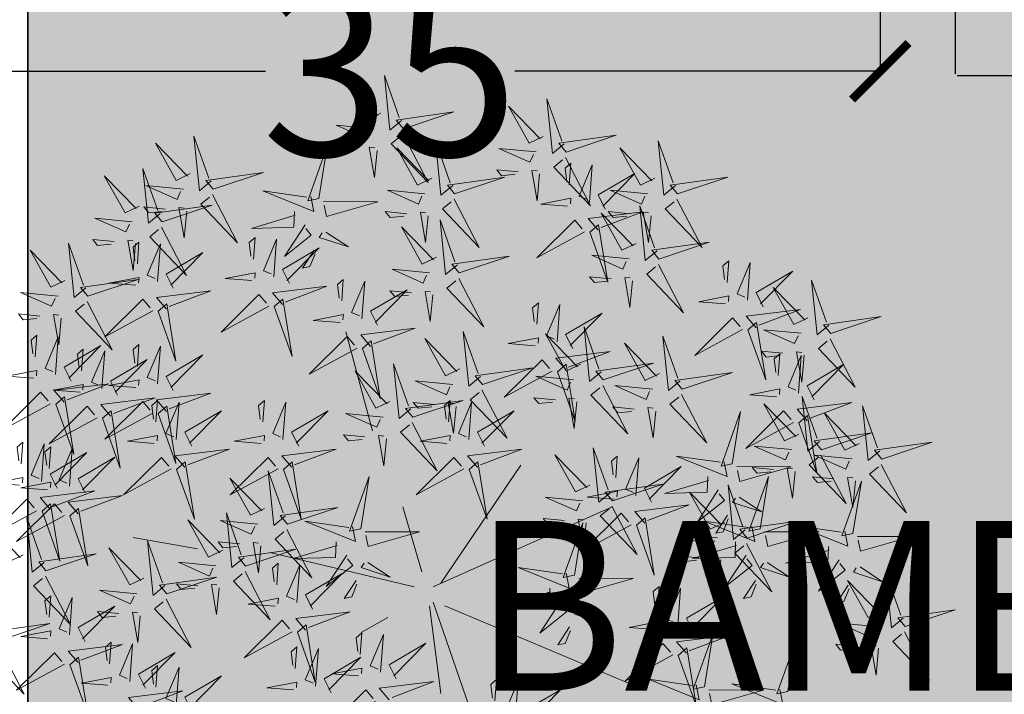
# Model space of a CAD drawing. Units: inches. Extents: x 1704 to 6393, y -157 to 1172.
# Tile 4 of 122: x 1898 to 1933, y 17 to 41. Entities that reach past the tile are written whole.
import ezdxf

# ---------------------------------------------------------------- set-up
doc = ezdxf.new("R2010")
doc.units = ezdxf.units.IN
doc.header["$MEASUREMENT"] = 0
for name, color, linetype, lineweight in [('A-ANNO-DIMS', 7, 'Continuous', 13), ('C-PROP', 7, 'Continuous', 35), ('L-shrub', 74, 'Continuous', 18), ('L-tree', 102, 'Continuous', 18)]:
    doc.layers.add(name, color=color, linetype=linetype, lineweight=lineweight)
doc.layers.add('L-PLNT-PATT', color=253, linetype='Continuous', lineweight=13, true_color=0x9abc8f)
doc.styles.get("Standard").update_dxf_attribs({"font": 'arial.ttf'})
doc.dimstyles.get("Standard").update_dxf_attribs({"dimtxt": 6, "dimasz": 2, "dimexe": 0.18, "dimexo": 0.0625, "dimgap": 0.09, "dimtad": 0, "dimtih": 1, "dimtoh": 1, "dimdec": 1, "dimzin": 0, "dimdsep": 46, "dimlunit": 3, "dimtxsty": 'Standard', "dimblk": 'ARCHTICK', "dimcen": 0.09, "dimadec": 0, "dimazin": 0, "dimtfac": 1, "dimtdec": 1, "dimtofl": 0, "dimtmove": 0, "dimatfit": 3, "dimfxl": 1, "dimtolj": 1, "dimtzin": 0, "dimarcsym": 0})

# ---------------------------------------------------------------- blocks, each defined once
blk = doc.blocks.new('bamboo')
at = {"layer": 'L-shrub'}
for p, q in [((43.5, 73), (278.2, 631.2)), ((-12.4, 39.5), (-247.1, 564.2)), ((-23.6, 61.9), (-370, 296.3)), ((32.3, 39.5), (390, 162.3)), ((43.5, 28.4), (300.5, 61.9)), ((-57.1, 6), (-247.1, -49.8)), ((-12.4, -16.3), (-113, -440.5)), ((77, -94.4), (121.7, -172.6)), ((-470.6, -139.1), (-761.2, -217.2)), ((-124.2, -652.6), (-157.7, -842.3))]:
    blk.add_line(p, q, dxfattribs=at)
for points in [[(103.7, 1424.7), (54.4, 1572.3), (77.9, 1403.4), (103.7, 1424.7)], [(-387.8, 1356.5), (-437.1, 1504.1), (-413.6, 1335.2), (-387.8, 1356.5)], [(119.4, 1423.2), (261.4, 1496.7), (147.9, 1388.7), (126.6, 1414.5)], [(-372, 1355), (-230.1, 1428.5), (-343.6, 1320.5), (-364.9, 1346.4)], [(-160.7, 1284.9), (-160, 1444.8), (-116.9, 1294.1), (-149.7, 1287.2)], [(79.4, 1419.1), (107.8, 1384.6), (-52.4, 1368.4), (70.8, 1412)], [(-756.4, 1206.5), (-805.8, 1354.1), (-782.2, 1185.2), (-756.4, 1206.5)], [(-412.1, 1350.9), (-383.7, 1316.4), (-543.9, 1300.2), (-420.7, 1343.8)], [(-70.9, 1292.4), (-27.7, 1358.5), (-55.4, 1272.9), (-68.6, 1281.5)], [(57.7, 1357.7), (77.5, 1316.1), (-31.5, 1255.3), (64.8, 1349.1)], [(103.3, 1337.4), (92.8, 1227.4), (133.3, 1318.7), (110.4, 1328.8)], [(167.7, 1347.1), (246.3, 1339.5), (157.6, 1324.2), (159.1, 1340)], [(-415.1, 1179.2), (-464.4, 1326.8), (-440.9, 1157.9), (-415.1, 1179.2)], [(-740.7, 1205), (-598.8, 1278.5), (-712.2, 1170.5), (-733.6, 1196.4)], [(-433.8, 1289.5), (-414, 1248), (-523, 1187.1), (-426.7, 1280.9)], [(-323.8, 1278.9), (-245.2, 1271.3), (-333.9, 1256.1), (-332.4, 1271.8)], [(-169.3, 1271.7), (-323, 1296.4), (-162.4, 1238.9), (-169.3, 1271.7)], [(161.7, 1284.2), (155.7, 1221.3), (172.9, 1235.5), (168.8, 1275.6)], [(-561.9, 1157.8), (-603.1, 1137.1), (-666.2, 1244.8), (-570.4, 1150.5)], [(-500.1, 1137.3), (-534, 1108.2), (-553.5, 1268), (-507.4, 1145.8)], [(-399.4, 1177.7), (-257.4, 1251.3), (-370.9, 1143.2), (-392.2, 1169.1)], [(-388.2, 1269.3), (-398.7, 1159.2), (-358.2, 1250.5), (-381.1, 1260.6)], [(-175.7, 1247.6), (-131.9, 1256.8), (-191.9, 1107.3), (-173.4, 1236.6)], [(-92.2, 1230.9), (0.4, 1170.5), (-61.7, 1248.7), (-81.3, 1233.2)], [(-18, 1257.9), (35, 1223.4), (30.4, 1245.3), (-7, 1260.2)], [(-329.8, 1216), (-335.8, 1153.1), (-318.6, 1167.3), (-322.7, 1207.4)], [(-780.7, 1200.9), (-752.3, 1166.4), (-912.5, 1150.2), (-789.3, 1193.8)], [(-131.4, 1199.8), (-85.3, 1198.1), (-81.9, 1073.4), (-120.4, 1202.1)], [(-439.4, 1173.7), (-411, 1139.2), (-571.2, 1122.9), (-448, 1166.6)], [(-494, 1113.1), (-347.5, 1165.5), (-515.9, 1138.5), (-494, 1113.1)], [(-174.3, 1012.2), (-173.7, 1172.1), (-130.6, 1021.4), (-163.4, 1014.5)], [(-802.5, 1139.6), (-782.6, 1098), (-891.6, 1037.1), (-795.3, 1130.9)], [(-692.4, 1128.9), (-613.8, 1121.3), (-702.5, 1106.1), (-701, 1121.8)], [(-773.2, 987.3), (-807.1, 958.2), (-826.6, 1118), (-780.4, 995.8)], [(-756.8, 1119.3), (-767.3, 1009.2), (-726.8, 1100.5), (-749.7, 1110.6)], [(-581.3, 1111.7), (-691.5, 1120), (-599.4, 1081.4), (-589.8, 1104.4)], [(-461.1, 1112.3), (-441.3, 1070.7), (-550.3, 1009.8), (-454, 1103.7)], [(-351.1, 1101.6), (-272.5, 1094), (-361.2, 1078.8), (-359.7, 1094.5)], [(-155.7, 961.1), (-205, 1108.7), (-181.5, 939.8), (-155.7, 961.1)], [(294.9, 1080.8), (141.2, 1105.5), (301.8, 1048), (294.9, 1080.8)], [(-835, 1007.8), (-876.2, 987.1), (-939.2, 1094.8), (-843.4, 1000.5)], [(-495.2, 1097.3), (-418.8, 957), (-529.1, 1068.2), (-503.7, 1090.1)], [(-415.5, 1092), (-426, 981.9), (-385.5, 1073.2), (-408.4, 1083.4)], [(-365.5, 930.4), (-364.8, 1090.2), (-321.7, 939.6), (-354.5, 932.7)], [(-84.5, 1019.7), (-41.3, 1085.8), (-69, 1000.1), (-82.2, 1008.8)], [(-698.4, 1066), (-704.4, 1003.1), (-687.2, 1017.3), (-691.3, 1057.4)], [(-633.3, 1052.3), (-696.3, 1057), (-681.8, 1040.1), (-641.8, 1045)], [(-570.3, 1047.5), (-576.3, 968.8), (-593.4, 1057.2), (-577.6, 1056)], [(288.5, 1056.7), (332.3, 1065.9), (272.3, 916.4), (290.8, 1045.7)], [(-767.1, 963.1), (-620.5, 1015.5), (-788.9, 988.5), (-767.1, 963.1)], [(-357.1, 1038.7), (-363.1, 975.8), (-345.9, 990), (-350, 1030.1)], [(-183, 999), (-336.7, 1023.7), (-176.1, 966.2), (-183, 999)], [(-140, 959.5), (2, 1033.1), (-111.5, 925), (-132.8, 950.9)], [(-275.7, 937.9), (-232.5, 1004), (-260.1, 918.3), (-273.4, 927)], [(-189.3, 974.8), (-145.6, 984), (-205.5, 834.6), (-187, 963.9)], [(-31.6, 985.2), (21.3, 950.7), (16.7, 972.5), (-20.7, 987.5)], [(289.9, 848.6), (290.5, 1008.4), (333.6, 857.8), (300.8, 850.9)], [(-854.3, 961.7), (-964.6, 970), (-872.5, 931.4), (-862.8, 954.4)], [(-180, 955.5), (-151.6, 921), (-311.8, 904.8), (-188.6, 948.4)], [(-105.9, 958.2), (-13.2, 897.8), (-75.4, 976), (-94.9, 960.5)], [(-768.3, 947.3), (-691.9, 807), (-802.2, 918.2), (-776.8, 940.1)], [(-374.1, 917.2), (-527.8, 941.9), (-367.2, 884.4), (-374.1, 917.2)], [(-145, 927.1), (-99, 925.4), (-95.6, 800.6), (-134.1, 929.4)], [(-1166, 756.5), (-1215.3, 904.1), (-1191.8, 735.2), (-1166, 756.5)], [(-906.4, 902.3), (-969.4, 907), (-954.8, 890.1), (-914.9, 895)], [(-843.4, 897.5), (-849.4, 818.8), (-866.4, 907.2), (-850.7, 906)], [(-592.6, 770.2), (-641.9, 917.8), (-618.4, 748.9), (-592.6, 770.2)], [(-380.5, 893), (-336.7, 902.2), (-396.6, 752.7), (-378.2, 882.1)], [(-222.7, 903.4), (-169.8, 868.9), (-174.4, 890.7), (-211.8, 905.7)], [(182.5, 782.8), (148.6, 753.6), (129.1, 913.5), (175.2, 791.2)], [(-297, 876.4), (-204.4, 816), (-266.5, 894.2), (-286.1, 878.7)], [(-201.7, 894.1), (-181.9, 852.5), (-290.9, 791.6), (-194.6, 885.5)], [(-156.1, 873.8), (-166.6, 763.7), (-126.1, 855), (-149, 865.2)], [(-91.7, 883.5), (-13.1, 875.8), (-101.8, 860.6), (-100.3, 876.4)], [(120.7, 803.3), (79.5, 782.6), (16.5, 890.3), (112.2, 796)], [(-974.8, 702), (-1024.2, 849.6), (-1000.7, 680.7), (-974.8, 702)], [(-576.8, 768.6), (-434.9, 842.2), (-548.4, 734.1), (-569.7, 760)], [(-336.2, 845.3), (-290.1, 843.6), (-286.7, 718.8), (-325.2, 847.6)], [(281.2, 835.4), (127.5, 860.1), (288.1, 802.6), (281.2, 835.4)], [(-1150.2, 755), (-1008.3, 828.6), (-1121.8, 720.5), (-1143.1, 746.4)], [(-97.7, 820.6), (-103.7, 757.7), (-86.5, 771.9), (-90.6, 811.9)], [(188.6, 758.6), (335.2, 810.9), (166.8, 784), (188.6, 758.6)], [(274.9, 811.2), (318.6, 820.4), (258.7, 670.9), (277.2, 800.3)], [(-199.8, 660.1), (-233.7, 630.9), (-253.2, 790.8), (-207, 668.5)], [(-959.1, 700.5), (-817.2, 774), (-930.7, 666), (-952, 691.8)], [(-616.9, 764.6), (-588.5, 730.1), (-748.7, 713.9), (-625.5, 757.5)], [(-261.6, 680.5), (-302.7, 659.9), (-365.8, 767.6), (-270, 673.2)], [(101.4, 757.2), (-8.9, 765.5), (83.2, 726.9), (92.9, 749.9)], [(-1190.3, 750.9), (-1161.9, 716.5), (-1322.1, 700.2), (-1198.9, 743.8)], [(187.4, 742.8), (263.8, 602.4), (153.5, 713.7), (178.9, 735.5)], [(-999.2, 696.4), (-970.7, 661.9), (-1131, 645.7), (-1007.8, 689.3)], [(-638.6, 703.2), (-618.8, 661.6), (-727.8, 600.7), (-631.5, 694.6)], [(-264.9, 565.6), (-314.3, 713.2), (-290.7, 544.3), (-264.9, 565.6)], [(49.3, 697.7), (-13.7, 702.5), (0.8, 685.5), (40.8, 690.4)], [(112.3, 693), (106.3, 614.2), (89.3, 702.6), (105, 701.5)], [(-1212, 689.6), (-1192.2, 648), (-1301.2, 587.1), (-1204.9, 680.9)], [(-1166.4, 669.3), (-1176.9, 559.2), (-1136.4, 650.5), (-1159.3, 660.7)], [(-1102, 678.9), (-1023.4, 671.3), (-1112.1, 656.1), (-1110.6, 671.8)], [(-619.9, 538.4), (-669.2, 686), (-645.7, 517), (-619.9, 538.4)], [(-593, 682.9), (-603.5, 572.8), (-563, 664.1), (-585.9, 674.3)], [(-528.6, 692.6), (-450, 684.9), (-538.7, 669.7), (-537.2, 685.5)], [(-193.7, 635.8), (-47.1, 688.2), (-215.5, 661.2), (-193.7, 635.8)], [(-1059.9, 523.7), (-1093.8, 494.6), (-1113.3, 654.4), (-1067.1, 532.2)], [(-280.9, 634.5), (-391.2, 642.7), (-299.1, 604.1), (-289.4, 627.2)], [(-249.2, 564.1), (-107.3, 637.7), (-220.7, 529.6), (-242.1, 555.5)], [(-1121.7, 544.2), (-1162.9, 523.5), (-1225.9, 631.2), (-1130.2, 536.9)], [(-1108, 616), (-1114, 553.1), (-1096.8, 567.3), (-1100.9, 607.4)], [(-1020.9, 635), (-1001.1, 593.4), (-1110, 532.6), (-1013.8, 626.4)], [(-975.2, 614.7), (-985.8, 504.7), (-945.3, 596), (-968.1, 606.1)], [(-910.8, 624.4), (-832.2, 616.8), (-921, 601.5), (-919.5, 617.3)], [(-604.1, 536.8), (-462.2, 610.4), (-575.7, 502.3), (-597, 528.2)], [(-534.6, 629.7), (-540.6, 566.8), (-523.4, 581), (-527.5, 621)], [(-194.9, 620.1), (-118.4, 479.7), (-228.8, 591), (-203.4, 612.8)], [(-37.8, 466.8), (-37.2, 626.6), (5.9, 476), (-26.9, 469.1)], [(-333, 575), (-396, 579.7), (-381.4, 562.8), (-341.5, 567.7)], [(-270, 570.3), (-276, 491.5), (-293, 579.9), (-277.2, 578.7)], [(-1288.8, 429.3), (-1338.2, 576.9), (-1314.7, 408), (-1288.8, 429.3)], [(-1053.8, 499.5), (-907.2, 551.9), (-1075.6, 524.9), (-1053.8, 499.5)], [(-916.9, 561.5), (-922.9, 498.6), (-905.6, 512.8), (-909.7, 552.9)], [(-650.3, 428.2), (-684.2, 399.1), (-703.7, 559), (-657.6, 436.7)], [(-289.2, 560), (-260.8, 525.6), (-421, 509.3), (-297.8, 552.9)], [(-712.1, 448.7), (-753.3, 428.1), (-816.4, 535.7), (-720.6, 441.4)], [(-644.2, 532.8), (-615.8, 498.3), (-776, 482), (-652.8, 525.7)], [(52, 474.3), (95.2, 540.4), (67.5, 454.7), (54.3, 463.3)], [(-1273.1, 427.7), (-1131.2, 501.3), (-1244.7, 393.3), (-1266, 419.1)], [(-1141, 498.1), (-1251.3, 506.4), (-1159.2, 467.8), (-1149.5, 490.8)], [(-311, 498.7), (-291.1, 457.1), (-400.1, 396.2), (-303.9, 490)], [(-1055, 483.7), (-978.6, 343.4), (-1088.9, 454.6), (-1063.5, 476.4)], [(-665.9, 471.4), (-646.1, 429.8), (-755.1, 368.9), (-658.8, 462.8)], [(-265.3, 478.4), (-275.8, 368.3), (-235.4, 459.6), (-258.2, 469.8)], [(-200.9, 488), (-122.3, 480.4), (-211, 465.2), (-209.5, 480.9)], [(-46.5, 453.6), (-200.1, 478.3), (-39.6, 420.8), (-46.5, 453.6)], [(-1193.1, 438.6), (-1256.1, 443.4), (-1241.5, 426.4), (-1201.6, 431.4)], [(-1130.1, 433.9), (-1136.1, 355.2), (-1153.1, 443.6), (-1137.4, 442.4)], [(-644.2, 404), (-497.6, 456.4), (-666, 429.4), (-644.2, 404)], [(-620.3, 451.1), (-630.8, 341), (-590.3, 432.3), (-613.2, 442.5)], [(-555.9, 460.7), (-477.3, 453.1), (-566, 437.9), (-564.5, 453.6)], [(-52.8, 429.4), (-9, 438.6), (-69, 289.1), (-50.5, 418.5)], [(104.9, 439.8), (157.9, 405.3), (153.3, 427.1), (115.9, 442.1)], [(-1313.2, 423.7), (-1284.7, 389.2), (-1445, 373), (-1321.8, 416.6)], [(-731.5, 402.7), (-841.7, 410.9), (-749.6, 372.3), (-739.9, 395.4)], [(-206.9, 425.1), (-212.9, 362.2), (-195.7, 376.4), (-199.8, 416.5)], [(30.7, 412.7), (123.3, 352.4), (61.2, 430.6), (41.6, 415)], [(393.8, 326), (352.6, 305.3), (289.5, 413), (385.3, 318.7)], [(-645.4, 388.3), (-569, 247.9), (-679.3, 359.1), (-653.9, 381)], [(-561.9, 397.8), (-567.9, 334.9), (-550.7, 349.1), (-554.8, 389.2)], [(-8.5, 381.7), (37.5, 380), (40.9, 255.2), (2.4, 384)], [(-1334.9, 362.3), (-1315.1, 320.7), (-1424, 259.8), (-1327.8, 353.7)], [(-1224.9, 351.7), (-1146.2, 344), (-1235, 328.8), (-1233.5, 344.6)], [(-783.5, 343.2), (-846.5, 347.9), (-832, 331), (-792, 335.9)], [(-720.5, 338.5), (-726.5, 259.7), (-743.5, 348.1), (-727.8, 346.9)], [(-1289.2, 342), (-1299.8, 231.9), (-1259.3, 323.3), (-1282.1, 333.4)], [(-606.2, 183.8), (-655.6, 331.4), (-632, 162.5), (-606.2, 183.8)], [(-363.6, 169.2), (-397.5, 140), (-417, 299.9), (-370.9, 177.6)], [(-1230.9, 288.8), (-1236.9, 225.9), (-1219.6, 240.1), (-1223.8, 280.1)], [(-933.9, 115.6), (-983.2, 263.3), (-959.7, 94.3), (-933.9, 115.6)], [(-425.4, 189.6), (-466.6, 169), (-529.7, 276.7), (-433.9, 182.4)], [(374.4, 279.9), (264.1, 288.2), (356.3, 249.6), (365.9, 272.6)], [(-1166, 102), (-1215.3, 249.6), (-1191.8, 80.7), (-1166, 102)], [(-590.5, 182.3), (-448.6, 255.9), (-562, 147.8), (-583.4, 173.7)], [(322.4, 220.5), (259.3, 225.2), (273.9, 208.3), (313.9, 213.2)], [(-1150.2, 100.5), (-1008.3, 174), (-1121.8, 66), (-1143.1, 91.9)], [(-918.2, 114.1), (-776.2, 187.7), (-889.7, 79.6), (-911, 105.5)], [(-630.5, 178.2), (-602.1, 143.7), (-762.3, 127.5), (-639.2, 171.1)], [(-357.5, 145), (-210.9, 197.3), (-379.3, 170.3), (-357.5, 145)], [(-444.7, 143.6), (-555, 151.8), (-462.9, 113.3), (-453.2, 136.3)], [(-652.3, 116.9), (-632.5, 75.3), (-741.4, 14.4), (-645.2, 108.2)], [(-510.6, -20.7), (-560, 126.9), (-536.5, -42), (-510.6, -20.7)], [(-358.7, 129.2), (-282.3, -11.2), (-392.6, 100.1), (-367.2, 121.9)], [(-1357.1, -48), (-1406.5, 99.6), (-1382.9, -69.3), (-1357.1, -48)], [(-1190.3, 96.4), (-1161.9, 61.9), (-1322.1, 45.7), (-1198.9, 89.3)], [(-958.2, 110.1), (-929.8, 75.6), (-1090, 59.3), (-966.8, 103)], [(-606.6, 96.6), (-617.1, -13.5), (-576.7, 77.8), (-599.5, 88)], [(-496.8, 84.1), (-559.8, 88.8), (-545.3, 71.9), (-505.3, 76.8)], [(-542.2, 106.2), (-463.6, 98.6), (-552.3, 83.4), (-550.8, 99.1)], [(-433.8, 79.4), (-439.8, 0.6), (-456.8, 89), (-441.1, 87.9)], [(-1212, 35.1), (-1192.2, -6.5), (-1301.2, -67.4), (-1204.9, 26.4)], [(-979.9, 48.7), (-960.1, 7.1), (-1069.1, -53.8), (-972.8, 40.1)], [(-869.9, 38), (-791.3, 30.4), (-880, 15.2), (-878.5, 30.9)], [(-548.2, 43.3), (-554.2, -19.6), (-537, -5.4), (-541.1, 34.7)], [(-494.9, -22.2), (-353, 51.3), (-466.5, -56.7), (-487.8, -30.9)], [(319, -89.9), (285.1, -119.1), (265.6, 40.8), (311.8, -81.4)], [(-1341.4, -49.5), (-1199.5, 24), (-1312.9, -84), (-1334.3, -58.1)], [(-1166.4, 14.8), (-1176.9, -95.3), (-1136.4, -4), (-1159.3, 6.1)], [(-1102, 24.4), (-1023.4, 16.8), (-1112.1, 1.6), (-1110.6, 17.3)], [(-934.3, 28.4), (-944.8, -81.7), (-904.3, 9.6), (-927.2, 19.8)], [(257.2, -69.4), (216.1, -90.1), (153, 17.6), (248.8, -76.7)], [(-875.9, -24.9), (-881.9, -87.8), (-864.7, -73.6), (-868.8, -33.5)], [(-718.6, -144.5), (-752.5, -173.6), (-772, -13.7), (-725.8, -136)], [(-535, -26.3), (-506.5, -60.8), (-666.8, -77), (-543.6, -33.4)], [(-174.3, -160.5), (-173.7, -0.6), (-130.6, -151.3), (-163.4, -158.2)], [(-1381.4, -53.6), (-1353, -88.1), (-1513.2, -104.3), (-1390.1, -60.7)], [(-1108, -38.5), (-1114, -101.4), (-1096.8, -87.2), (-1100.9, -47.1)], [(-780.4, -124), (-821.5, -144.7), (-884.6, -37), (-788.8, -131.3)], [(-1403.2, -114.9), (-1383.3, -156.5), (-1492.3, -217.4), (-1396.1, -123.6)], [(-556.7, -87.7), (-536.9, -129.3), (-645.8, -190.1), (-549.6, -96.3)], [(-511, -108), (-521.6, -218), (-481.1, -126.7), (-503.9, -116.6)], [(-446.7, -98.3), (-368, -105.9), (-456.8, -121.2), (-455.3, -105.4)], [(-84.5, -153), (-41.3, -86.9), (-69, -172.5), (-82.2, -163.9)], [(237.9, -115.5), (127.6, -107.2), (219.7, -145.8), (229.4, -122.8)], [(-1357.5, -135.2), (-1368, -245.3), (-1327.6, -154), (-1350.4, -143.9)], [(-1293.1, -125.6), (-1214.5, -133.2), (-1303.2, -148.4), (-1301.7, -132.7)], [(-1143.7, -283.2), (-1143, -123.3), (-1099.9, -274), (-1132.7, -280.9)], [(-712.5, -168.7), (-565.9, -116.3), (-734.3, -143.3), (-712.5, -168.7)], [(323.9, -129.9), (400.4, -270.3), (290, -159), (315.4, -137.2)], [(-799.7, -170.1), (-910, -161.8), (-817.9, -200.4), (-808.2, -177.3)], [(-452.7, -161.2), (-458.7, -224.1), (-441.4, -209.9), (-445.5, -169.8)], [(-183, -173.7), (-336.7, -149), (-176.1, -206.5), (-183, -173.7)], [(185.8, -175), (122.8, -170.2), (137.4, -187.2), (177.4, -182.3)], [(298.2, -260.3), (257, -281), (193.9, -173.3), (289.7, -267.6)], [(248.8, -179.7), (242.8, -258.4), (225.8, -170), (241.6, -171.2)], [(-1299.1, -188.5), (-1305.1, -251.4), (-1287.9, -237.2), (-1292, -197.1)], [(-713.7, -184.4), (-637.3, -324.8), (-747.6, -213.6), (-722.2, -191.7)], [(-189.3, -197.8), (-145.6, -188.6), (-205.5, -338.1), (-187, -208.8)], [(-105.9, -214.5), (-13.2, -274.9), (-75.4, -196.7), (-94.9, -212.2)], [(-31.6, -187.5), (21.3, -222), (16.7, -200.1), (-20.7, -185.2)], [(-1053.9, -275.7), (-1010.7, -209.6), (-1038.4, -295.3), (-1051.6, -286.6)], [(-851.8, -229.5), (-914.8, -224.8), (-900.2, -241.7), (-860.3, -236.8)], [(-788.8, -234.2), (-794.8, -313), (-811.8, -224.6), (-796, -225.8)], [(52.5, -314.9), (11.3, -335.6), (-51.8, -227.9), (44, -322.2)], [(114.3, -335.4), (80.4, -364.5), (60.9, -204.6), (107, -326.9)], [(-363.6, -376.3), (-397.5, -405.4), (-417, -245.5), (-370.9, -367.8)], [(-196.6, -388.9), (-246, -241.3), (-222.5, -410.2), (-196.6, -388.9)], [(-145, -245.6), (-99, -247.3), (-95.6, -372), (-134.1, -243.3)], [(-1152.3, -296.4), (-1306, -271.7), (-1145.4, -329.2), (-1152.3, -296.4)], [(-841.4, -403.5), (-875.3, -432.7), (-894.8, -272.8), (-848.7, -395.1)], [(-425.4, -355.8), (-466.6, -376.5), (-529.7, -268.8), (-433.9, -363.1)], [(-1158.7, -320.6), (-1114.9, -311.4), (-1174.8, -460.8), (-1156.4, -331.5)], [(-903.2, -383.1), (-944.4, -403.7), (-1007.5, -296), (-911.7, -390.3)], [(-1000.9, -310.2), (-948, -344.7), (-952.6, -322.9), (-990, -307.9)], [(-180.9, -390.4), (-39, -316.9), (-152.5, -424.9), (-173.8, -399)], [(120.3, -359.6), (266.9, -307.2), (98.5, -334.2), (120.3, -359.6)], [(278.8, -306.4), (168.6, -298.1), (260.7, -336.7), (270.4, -313.7)], [(-1075.2, -337.2), (-982.6, -397.6), (-1044.7, -319.4), (-1064.3, -334.9)], [(-1114.4, -368.3), (-1068.3, -370), (-1064.9, -494.8), (-1103.4, -366)], [(-835.4, -427.8), (-688.8, -375.4), (-857.2, -402.4), (-835.4, -427.8)], [(-357.5, -400.5), (-210.9, -348.1), (-379.3, -375.1), (-357.5, -400.5)], [(-73.8, -511.6), (-123.1, -364), (-99.6, -532.9), (-73.8, -511.6)], [(33.1, -361), (-77.2, -352.7), (14.9, -391.3), (24.6, -368.2)], [(119.1, -375.3), (195.6, -515.7), (85.2, -404.5), (110.7, -382.6)], [(226.8, -365.9), (163.8, -361.1), (178.3, -378.1), (218.3, -373.2)], [(289.8, -370.6), (283.8, -449.3), (266.8, -360.9), (282.5, -362.1)], [(-444.7, -401.9), (-555, -393.6), (-462.9, -432.2), (-453.2, -409.1)], [(-221, -394.5), (-192.5, -429), (-352.8, -445.2), (-229.6, -401.6)], [(-922.6, -429.1), (-1032.9, -420.9), (-940.7, -459.5), (-931.1, -436.4)], [(-358.7, -416.2), (-282.3, -556.6), (-392.6, -445.4), (-367.2, -423.5)], [(-19, -420.4), (-82, -415.7), (-67.4, -432.6), (-27.4, -427.7)], [(44, -425.1), (38, -503.9), (21, -415.5), (36.8, -416.7)], [(-1179.6, -607.1), (-1229, -459.4), (-1205.5, -628.4), (-1179.6, -607.1)], [(-836.6, -443.5), (-760.1, -583.9), (-870.5, -472.6), (-845, -450.8)], [(-496.8, -461.3), (-559.8, -456.6), (-545.3, -473.5), (-505.3, -468.6)], [(-433.8, -466), (-439.8, -544.8), (-456.8, -456.4), (-441.1, -457.6)], [(-242.7, -455.8), (-222.9, -497.4), (-331.8, -558.3), (-235.6, -464.5)], [(-58, -513.1), (83.9, -439.6), (-29.6, -547.6), (-50.9, -521.7)], [(-974.6, -488.6), (-1037.7, -483.9), (-1023.1, -500.8), (-983.1, -495.9)], [(-911.6, -493.3), (-917.6, -572.1), (-934.7, -483.7), (-918.9, -484.8)], [(-197, -476.1), (-207.5, -586.2), (-167.1, -494.9), (-189.9, -484.8)], [(-132.6, -466.5), (-54, -474.1), (-142.8, -489.3), (-141.3, -473.6)], [(-98.1, -517.2), (-69.7, -551.7), (-229.9, -567.9), (-106.7, -524.3)], [(-1163.9, -608.6), (-1022, -535), (-1135.5, -643.1), (-1156.8, -617.2)], [(-138.6, -529.4), (-144.7, -592.3), (-127.4, -578.1), (-131.5, -538)], [(-363.6, -689.9), (-397.5, -719), (-417, -559.2), (-370.9, -681.4)], [(-425.4, -669.4), (-466.6, -690.1), (-529.7, -582.4), (-433.9, -676.7)], [(-119.8, -578.6), (-100, -620.2), (-209, -681), (-112.7, -587.2)], [(-74.2, -598.9), (-84.7, -708.9), (-44.2, -617.6), (-67, -607.5)], [(8.2, -743.4), (-41.2, -595.8), (-17.7, -764.7), (8.2, -743.4)], [(-9.8, -589.2), (68.8, -596.8), (-19.9, -612), (-18.4, -596.3)], [(352.8, -669.4), (311.6, -690.1), (248.5, -582.4), (344.3, -676.7)], [(-1204, -612.6), (-1175.5, -647.1), (-1335.8, -663.4), (-1212.6, -619.7)], [(-1084.1, -757), (-1133.4, -609.4), (-1109.9, -778.4), (-1084.1, -757)], [(-827.8, -744.4), (-861.7, -773.6), (-881.2, -613.7), (-835.1, -736)], [(-527.4, -744.4), (-561.3, -773.6), (-580.8, -613.7), (-534.7, -736)], [(-889.6, -724), (-930.8, -744.6), (-993.8, -636.9), (-898.1, -731.2)], [(-589.2, -724), (-630.4, -744.6), (-693.5, -636.9), (-597.7, -731.2)], [(-357.5, -714.1), (-210.9, -661.7), (-379.3, -688.7), (-357.5, -714.1)], [(-15.8, -652.1), (-21.8, -715), (-4.6, -700.8), (-8.7, -660.7)], [(-1225.7, -674), (-1205.9, -715.6), (-1314.8, -776.5), (-1218.6, -682.6)], [(-1115.6, -684.7), (-1037, -692.3), (-1125.7, -707.5), (-1124.2, -691.8)], [(-1068.3, -758.6), (-926.4, -685), (-1039.9, -793.1), (-1061.2, -767.2)], [(23.9, -744.9), (165.8, -671.4), (52.3, -779.4), (31, -753.6)], [(-1180, -694.3), (-1190.5, -804.4), (-1150.1, -713.1), (-1172.9, -702.9)], [(-821.7, -768.6), (-675.1, -716.3), (-843.5, -743.3), (-821.7, -768.6)], [(-444.7, -715.5), (-555, -707.2), (-462.9, -745.8), (-453.2, -722.8)], [(-521.3, -768.6), (-374.8, -716.3), (-543.2, -743.3), (-521.3, -768.6)], [(284.5, -805.8), (243.4, -826.4), (180.3, -718.7), (276.1, -813.1)], [(333.5, -715.5), (223.2, -707.2), (315.3, -745.8), (325, -722.8)], [(346.4, -826.2), (312.4, -855.4), (293, -695.5), (339.1, -817.8)], [(-1121.6, -747.6), (-1127.7, -810.5), (-1110.4, -796.3), (-1114.5, -756.2)], [(-358.7, -729.9), (-282.3, -870.2), (-392.6, -759), (-367.2, -737.1)], [(-16.2, -749), (12.3, -783.5), (-148, -799.7), (-24.8, -756.1)], [(-1108.4, -762.6), (-1079.9, -797.1), (-1240.2, -813.4), (-1117, -769.7)], [(-908.9, -770), (-1019.2, -761.8), (-927.1, -800.3), (-917.4, -777.3)], [(-608.6, -770), (-718.8, -761.8), (-626.7, -800.3), (-617.1, -777.3)], [(-513.8, -908.1), (-547.7, -937.2), (-567.2, -777.3), (-521, -899.6)], [(-496.8, -774.9), (-559.8, -770.2), (-545.3, -787.1), (-505.3, -782.2)], [(-433.8, -779.7), (-439.8, -858.4), (-456.8, -770), (-441.1, -771.2)], [(281.4, -774.9), (218.4, -770.2), (232.9, -787.1), (272.9, -782.2)], [(-822.9, -784.4), (-746.5, -924.8), (-856.8, -813.5), (-831.4, -791.7)], [(-575.6, -887.6), (-616.8, -908.3), (-679.8, -800.6), (-584, -894.9)], [(-522.5, -784.4), (-446.1, -924.8), (-556.4, -813.5), (-531, -791.7)], [(-1130.1, -824), (-1110.3, -865.6), (-1219.3, -926.5), (-1123, -832.6)], [(-1020.1, -834.7), (-941.4, -842.3), (-1030.2, -857.5), (-1028.7, -841.8)], [(-961, -829.5), (-1024, -824.8), (-1009.5, -841.7), (-969.5, -836.8)], [(-898, -834.2), (-904, -913), (-921, -824.6), (-905.3, -825.7)], [(-865.6, -975.2), (-915, -827.6), (-891.5, -996.5), (-865.6, -975.2)], [(-660.6, -829.5), (-723.6, -824.8), (-709.1, -841.7), (-669.1, -836.8)], [(-597.6, -834.2), (-603.6, -913), (-620.7, -824.6), (-604.9, -825.7)], [(-37.9, -810.4), (-18.1, -852), (-127, -912.8), (-30.8, -819)], [(7.8, -830.7), (-2.8, -940.7), (37.7, -849.4), (14.9, -839.3)], [(72.2, -821), (150.8, -828.6), (62, -843.8), (63.5, -828.1)], [(-1084.5, -844.3), (-1095, -954.4), (-1054.5, -863.1), (-1077.3, -852.9)], [(265.2, -851.8), (154.9, -843.6), (247, -882.2), (256.7, -859.1)], [(-507.7, -932.3), (-361.1, -879.9), (-529.5, -906.9), (-507.7, -932.3)], [(-288.9, -983), (-330, -1003.7), (-393.1, -896), (-297.3, -990.3)], [(-227.1, -1003.5), (-261, -1032.7), (-280.5, -872.8), (-234.3, -995)], [(148, -983), (106.8, -1003.7), (43.8, -896), (139.5, -990.3)], [(66.1, -883.9), (60.1, -946.8), (77.4, -932.6), (73.3, -892.5)], [(209.8, -1003.5), (175.9, -1032.7), (156.4, -872.8), (202.6, -995)], [(-1026.1, -897.6), (-1032.1, -960.5), (-1014.9, -946.3), (-1019, -906.2)], [(-849.9, -976.7), (-708, -903.2), (-821.4, -1011.2), (-842.8, -985.4)], [(-554.7, -1044.4), (-588.6, -1073.6), (-608.1, -913.7), (-562, -1036)], [(213.1, -911.3), (150.1, -906.6), (164.7, -923.5), (204.7, -918.6)], [(276.1, -916), (270.1, -994.8), (253.1, -906.4), (268.9, -907.6)], [(-616.5, -1023.9), (-657.7, -1044.6), (-720.8, -936.9), (-625, -1031.2)], [(-594.9, -933.7), (-705.2, -925.4), (-613.1, -964), (-603.4, -940.9)], [(-508.9, -948), (-432.5, -1088.4), (-542.8, -977.2), (-517.4, -955.3)], [(-60.1, -1097.9), (-109.5, -950.3), (-85.9, -1119.2), (-60.1, -1097.9)], [(-889.9, -980.8), (-861.5, -1015.3), (-1021.7, -1031.5), (-898.6, -987.9)], [(-302.5, -1064.9), (-343.7, -1085.5), (-406.8, -977.8), (-311, -1072.1)], [(-240.7, -1085.3), (-274.6, -1114.5), (-294.1, -954.6), (-248, -1076.9)], [(-221, -1027.7), (-74.4, -975.4), (-242.8, -1002.3), (-221, -1027.7)], [(215.9, -1027.7), (362.5, -975.4), (194.1, -1002.3), (215.9, -1027.7)], [(-647, -993.1), (-710, -988.4), (-695.4, -1005.3), (-655.5, -1000.4)], [(-584, -997.8), (-590, -1076.6), (-607, -988.2), (-591.3, -989.4)], [(-548.6, -1068.6), (-402.1, -1016.3), (-570.5, -1043.2), (-548.6, -1068.6)], [(-308.2, -1029.1), (-418.5, -1020.8), (-326.4, -1059.4), (-316.7, -1036.4)], [(-44.4, -1099.5), (97.5, -1025.9), (-15.9, -1134), (-37.3, -1108.1)], [(128.7, -1029.1), (18.4, -1020.8), (110.5, -1059.4), (120.2, -1036.4)], [(-911.7, -1042.2), (-891.9, -1083.8), (-1000.8, -1144.6), (-904.6, -1050.8)], [(-866, -1062.5), (-876.5, -1172.5), (-836.1, -1081.2), (-858.9, -1071.1)], [(-801.6, -1052.8), (-723, -1060.4), (-811.7, -1075.7), (-810.2, -1059.9)], [(-635.9, -1070), (-746.1, -1061.7), (-654, -1100.3), (-644.4, -1077.3)], [(-234.6, -1109.5), (-88.1, -1057.2), (-256.5, -1084.1), (-234.6, -1109.5)], [(-222.2, -1043.5), (-145.8, -1183.9), (-256.1, -1072.6), (-230.7, -1050.8)], [(214.7, -1043.5), (291.1, -1183.9), (180.8, -1072.6), (206.2, -1050.8)], [(-549.8, -1084.4), (-473.4, -1224.8), (-583.8, -1113.5), (-558.3, -1091.7)], [(-360.3, -1088.6), (-423.3, -1083.8), (-408.7, -1100.8), (-368.8, -1095.8)], [(-297.3, -1093.3), (-303.3, -1172), (-320.3, -1083.6), (-304.5, -1084.8)], [(76.6, -1088.6), (13.6, -1083.8), (28.1, -1100.8), (68.1, -1095.8)], [(144.7, -1234.3), (95.3, -1086.7), (118.8, -1255.6), (144.7, -1234.3)], [(139.6, -1093.3), (133.6, -1172), (116.6, -1083.6), (132.3, -1084.8)], [(-807.6, -1115.7), (-813.6, -1178.6), (-796.4, -1164.4), (-800.5, -1124.4)], [(-687.9, -1129.5), (-751, -1124.7), (-736.4, -1141.7), (-696.4, -1136.8)], [(-624.9, -1134.2), (-630.9, -1213), (-648, -1124.6), (-632.2, -1125.7)], [(-321.9, -1110.9), (-432.1, -1102.7), (-340, -1141.2), (-330.3, -1118.2)], [(-235.8, -1125.3), (-159.4, -1265.7), (-269.7, -1154.4), (-244.3, -1132.6)], [(-84.4, -1103.5), (-56, -1138), (-216.2, -1154.2), (-93.1, -1110.6)], [(-373.9, -1170.4), (-436.9, -1165.7), (-422.4, -1182.6), (-382.4, -1177.7)], [(-310.9, -1175.1), (-316.9, -1253.9), (-334, -1165.5), (-318.2, -1166.6)], [(-106.2, -1164.9), (-86.3, -1206.5), (-195.3, -1267.4), (-99.1, -1173.5)], [(160.4, -1235.8), (302.3, -1162.3), (188.8, -1270.3), (167.5, -1244.4)]]:
    blk.add_lwpolyline(points, dxfattribs=at)
blk = doc.blocks.new('_ArchTick')
at = {"color": 0, "linetype": 'ByBlock', "const_width": 0.15}
blk.add_lwpolyline([(-0.5, -0.5), (0.5, 0.5)], dxfattribs=at)
blk = doc.blocks.new('*D70')
at = {"layer": 'A-ANNO-DIMS', "color": 0, "lineweight": -2, "transparency": 16777216}
for p, q in [((1931.245, 38.926), (1936.991, 38.926)), ((1936.811, 38.926), (1936.811, 23.36)), ((1936.811, 1.402), (1936.811, 16.968)), ((1931.245, 1.402), (1936.991, 1.402))]:
    blk.add_line(p, q, dxfattribs=at)
at = {"layer": 'Defpoints', "color": 0, "lineweight": -3, "transparency": 16777216}
for p in [(1931.183, 38.926), (1931.183, 1.402), (1936.811, 1.402)]:
    blk.add_point(p, dxfattribs=at)
at = {"layer": 'A-ANNO-DIMS', "color": 0, "lineweight": -2, "transparency": 16777216, "xscale": 2, "yscale": 2, "zscale": 2}
for p, rotation in [((1936.811, 38.926), 90), ((1936.811, 1.402), 270)]:
    blk.add_blockref('_ArchTick', p, dxfattribs=dict(at, rotation=rotation))
at = {"layer": 'A-ANNO-DIMS', "color": 0, "transparency": 16777216, "insert": (1936.811, 20.164), "char_height": 6, "attachment_point": 5}
blk.add_mtext('\\A1;BAMBOO 38', dxfattribs=at)
blk = doc.blocks.new('*D71')
at = {"layer": 'A-ANNO-DIMS', "color": 0, "lineweight": -2, "transparency": 16777216}
for p, q in [((1894.896, 38.988), (1894.896, 44.734)), ((1931.183, 38.988), (1931.183, 44.734)), ((1894.896, 44.554), (1908.656, 44.554)), ((1931.183, 44.554), (1917.422, 44.554))]:
    blk.add_line(p, q, dxfattribs=at)
at = {"layer": 'Defpoints', "color": 0, "lineweight": -3, "transparency": 16777216}
for p in [(1931.183, 44.554), (1894.896, 38.926), (1931.183, 38.926)]:
    blk.add_point(p, dxfattribs=at)
at = {"layer": 'A-ANNO-DIMS', "color": 0, "lineweight": -2, "transparency": 16777216, "xscale": 2, "yscale": 2, "zscale": 2, "rotation": 180}
blk.add_blockref('_ArchTick', (1894.896, 44.554), dxfattribs=at)
at = {"layer": 'A-ANNO-DIMS', "color": 0, "lineweight": -2, "transparency": 16777216, "xscale": 2, "yscale": 2, "zscale": 2}
blk.add_blockref('_ArchTick', (1931.183, 44.554), dxfattribs=at)
at = {"layer": 'A-ANNO-DIMS', "color": 0, "transparency": 16777216, "insert": (1913.039, 44.554), "char_height": 6, "attachment_point": 5}
blk.add_mtext('\\A1;36', dxfattribs=at)
blk = doc.blocks.new('*D87')
at = {"layer": 'A-ANNO-DIMS', "color": 0, "lineweight": -2, "transparency": 16777216}
for p, q in [((1893.829, 44.479), (1893.829, 38.903)), ((1928.523, 44.479), (1928.523, 38.903)), ((1893.829, 39.083), (1906.768, 39.083)), ((1928.523, 39.083), (1915.584, 39.083))]:
    blk.add_line(p, q, dxfattribs=at)
at = {"layer": 'Defpoints', "color": 0, "lineweight": -3, "transparency": 16777216}
for p in [(1893.829, 44.542), (1928.523, 44.542), (1928.523, 39.083)]:
    blk.add_point(p, dxfattribs=at)
at = {"layer": 'A-ANNO-DIMS', "color": 0, "lineweight": -2, "transparency": 16777216, "xscale": 2, "yscale": 2, "zscale": 2, "rotation": 180}
blk.add_blockref('_ArchTick', (1893.829, 39.083), dxfattribs=at)
at = {"layer": 'A-ANNO-DIMS', "color": 0, "lineweight": -2, "transparency": 16777216, "xscale": 2, "yscale": 2, "zscale": 2}
blk.add_blockref('_ArchTick', (1928.523, 39.083), dxfattribs=at)
at = {"layer": 'A-ANNO-DIMS', "color": 0, "transparency": 16777216, "insert": (1911.176, 39.083), "char_height": 6, "attachment_point": 5}
blk.add_mtext('\\A1;35', dxfattribs=at)

msp = doc.modelspace()

# ---------------------------------------------------------------- hatches: boundary and pattern name
at = {"layer": 'L-PLNT-PATT', "transparency": 33554643}
h = msp.add_hatch(color=256, dxfattribs=at)
h.dxf.hatch_style = 1
h.paths.add_polyline_path([(1975.349, 202.213), (1898.349, 202.213), (1898.349, -3.787), (1975.349, -3.787)])

# ---------------------------------------------------------------- linework, layer by layer
at = {"layer": 'C-PROP'}
msp.add_line((1898.349, -3.787), (1898.349, 1033.213), dxfattribs=at)

# ---------------------------------------------------------------- block references
at = {"layer": 'L-tree', "xscale": 0.0120554306156665, "yscale": 0.0120554306156665, "zscale": 0.0120554306156665, "rotation": 270}
msp.add_blockref('bamboo', (1912.228, 20.683), dxfattribs=at)

# ---------------------------------------------------------------- dimensions: what is measured, and where the dimension line sits
at = {"layer": 'A-ANNO-DIMS'}
for base, p1, p2, picture, middle in [((1931.183, 44.554), (1894.896, 38.926), (1931.183, 38.926), '*D71', (1913.039, 44.554)), ((1928.523, 39.083), (1893.829, 44.542), (1928.523, 44.542), '*D87', (1911.176, 39.083))]:
    dim = msp.add_linear_dim(base=base, p1=p1, p2=p2, dimstyle='Standard', override={"dimdec": 0, "dimlfac": 1, "dimrnd": 0, "dimzin": 0, "dimdsep": 46, "dimlunit": 2}, dxfattribs=at)
    dim.commit()
    dim.dimension.update_dxf_attribs({"geometry": picture, "text_midpoint": middle})
dim = msp.add_linear_dim(base=(1936.811, 1.402), p1=(1931.183, 38.926), p2=(1931.183, 1.402), angle=270, text='BAMBOO <>', dimstyle='Standard', override={"dimdec": 0, "dimlfac": 1, "dimrnd": 0, "dimzin": 0, "dimdsep": 46, "dimlunit": 2}, dxfattribs=at)
dim.commit()
dim.dimension.update_dxf_attribs({"geometry": '*D70', "text_midpoint": (1936.811, 20.164)})

doc.saveas('drawing.dxf')
